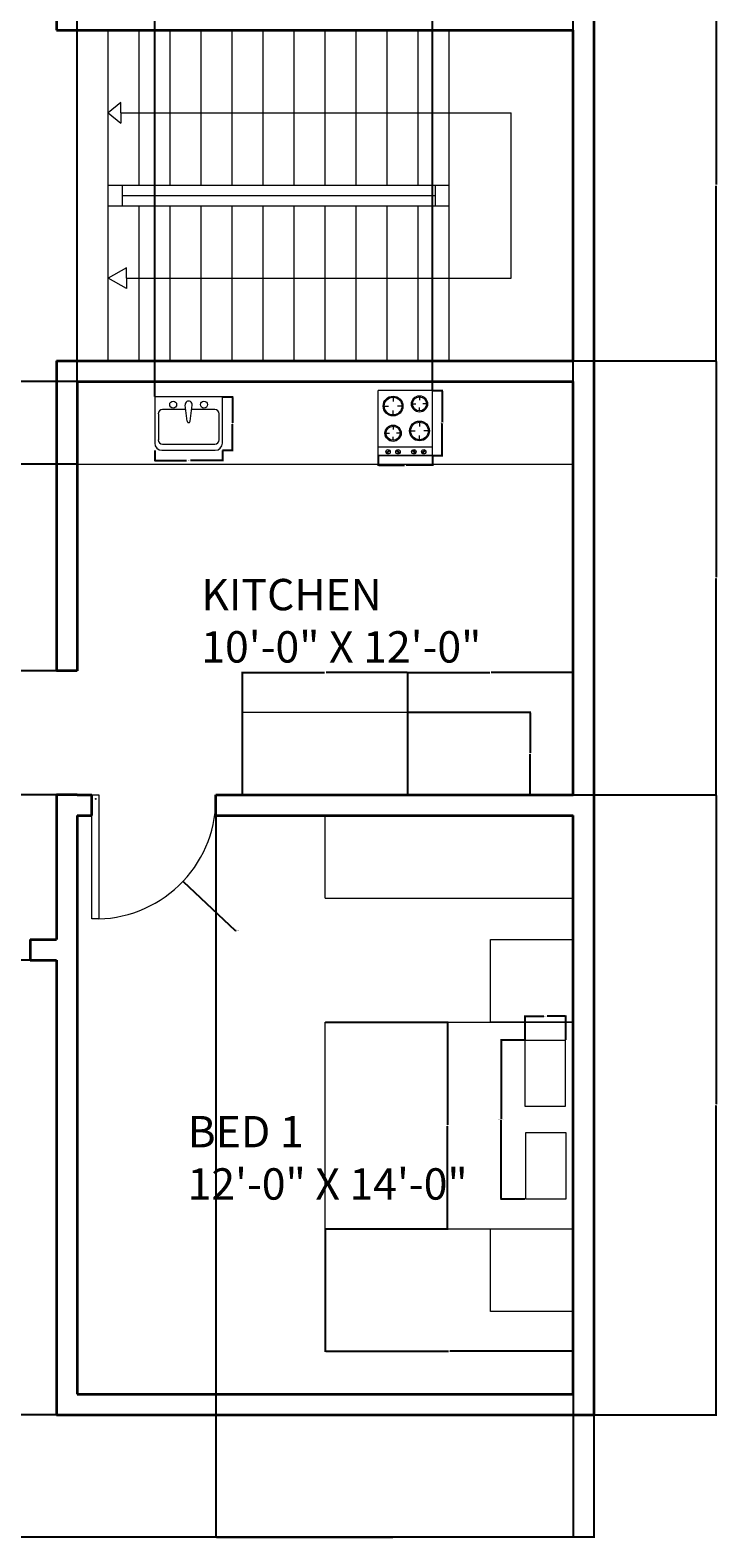
# Model space of a CAD drawing. Units: inches. Extents: x 4468 to 4972, y 2758 to 3538.
# Tile 2 of 4: x 4772 to 4972, y 2758 to 3196. Entities that reach past the tile are written whole.
import ezdxf

# ---------------------------------------------------------------- set-up
doc = ezdxf.new("R2010")
doc.units = ezdxf.units.IN
for name, color, linetype, lineweight in [('A-ANNO-DIMS', 2, 'Continuous', 18), ('A-AREA-IDEN', 7, 'Continuous', 18), ('A-DOOR', 4, 'Continuous', 18), ('A-EQPM', 8, 'Continuous', 18), ('A-FLOR-CASE', 9, 'Continuous', 18), ('A-FLOR-FIXT', 9, 'Continuous', 18), ('A-FLOR-STRS', 3, 'Continuous', 18), ('A-FURN', 8, 'Continuous', 15), ('A-WALL', 7, 'Continuous', 35)]:
    doc.layers.add(name, color=color, linetype=linetype, lineweight=lineweight)
doc.styles.get("Standard").update_dxf_attribs({"font": 'arial.ttf'})
doc.dimstyles.get("Standard").update_dxf_attribs({"dimtxt": 0.18, "dimasz": 0.18, "dimexe": 0.18, "dimexo": 0.0625, "dimgap": 0.09, "dimtad": 0, "dimtih": 1, "dimtoh": 1, "dimdec": 4, "dimzin": 0, "dimdsep": 46, "dimtxsty": 'Standard', "dimcen": 0.09, "dimadec": 0, "dimazin": 0, "dimtfac": 1, "dimtdec": 4, "dimtofl": 0, "dimtmove": 0, "dimatfit": 3, "dimfxl": 1, "dimtolj": 1, "dimtzin": 0, "dimarcsym": 0})

# ---------------------------------------------------------------- blocks, each defined once
blk = doc.blocks.new('A$C16A60262')
at = {"linetype": 'ByBlock'}
for p, q in [((0, 600), (0, 0)), ((488, 600), (0, 600)), ((0, 600), (500, 600)), ((0, 600), (500, 600)), ((500, 600), (500, 0)), ((500, 600), (500, 0)), ((500, 520), (0, 520)), ((119, 456), (119, 415)), ((363, 460), (363, 427)), ((38, 374), (79, 374)), ((119, 293), (119, 334)), ((201, 374), (160, 374)), ((298, 395), (331, 395)), ((363, 330), (363, 362)), ((428, 395), (396, 395)), ((119, 189), (119, 156)), ((282, 144), (323, 144)), ((363, 225), (363, 185)), ((445, 144), (404, 144)), ((0, 0), (500, 0)), ((54, 124), (87, 124)), ((119, 59), (119, 91)), ((184, 124), (152, 124)), ((363, 63), (363, 103))]:
    blk.add_line(p, q, dxfattribs=at)
for p, q in [((66, 557), (87, 579)), ((72, 552), (66, 557)), ((93, 573), (72, 552)), ((87, 579), (93, 573)), ((158, 572), (163, 578)), ((179, 551), (158, 572)), ((163, 578), (184, 557)), ((184, 557), (179, 551)), ((305, 572), (311, 578)), ((326, 551), (305, 572)), ((311, 578), (332, 557)), ((332, 557), (326, 551)), ((396, 558), (417, 580)), ((402, 553), (396, 558)), ((423, 574), (402, 553)), ((417, 580), (423, 574))]:
    blk.add_line(p, q)
for centre in [(80, 566), (171, 566), (318, 566), (409, 566)]:
    blk.add_circle(centre, 20.6)
for centre, radius in [((119, 374), 91.3), ((119, 374), 81.3), ((363, 395), 75), ((363, 395), 65), ((119, 124), 75), ((119, 124), 65), ((363, 144), 91.3), ((363, 144), 81.3)]:
    blk.add_circle(centre, radius, dxfattribs=at)
blk = doc.blocks.new('A$C34D52403')
for p, q in [((0, 0.457), (0, 0.061)), ((0.579, 0.457), (0, 0.457)), ((0.277, 0.249), (0.26, 0.387)), ((0.302, 0.249), (0.319, 0.387)), ((0.579, 0.061), (0.579, 0.457)), ((0.031, 0.312), (0.031, 0.089)), ((0.266, 0.349), (0.068, 0.349)), ((0.513, 0.349), (0.313, 0.349)), ((0.55, 0.089), (0.55, 0.312)), ((0.068, 0.052), (0.513, 0.052)), ((0.061, 0), (0.518, 0))]:
    blk.add_line(p, q)
for centre in [(0.158, 0.391), (0.421, 0.391)]:
    blk.add_circle(centre, 0.0296)
for centre, radius, start, end in [((0.29, 0.391), 0.0296, 353.0422, 186.9578), ((0.068, 0.312), 0.0371, 90, 180), ((0.513, 0.312), 0.0371, 0, 90), ((0.29, 0.249), 0.0125, 179.3528, 0.6472), ((0.061, 0.061), 0.061, 180, 270), ((0.068, 0.089), 0.0371, 180, 270), ((0.513, 0.089), 0.0371, 270, 0), ((0.518, 0.061), 0.061, 270, 0)]:
    blk.add_arc(centre, radius, start, end)
blk = doc.blocks.new('DOOR-LEAF-36IN')
for p, q in [((0, 0), (0, 36)), ((0, 36), (2, 36)), ((2, 36), (2, 0)), ((2, 0), (0, 0))]:
    blk.add_line(p, q)
blk = doc.blocks.new('BED-PILLOW-PAIR')
for points in [[(0, 46.15), (11.65, 46.15), (11.65, 26.85), (0, 26.85)], [(0.18, 19.3), (11.83, 19.3), (11.83, 0), (0.18, 0)]]:
    blk.add_lwpolyline(points, close=True)
blk = doc.blocks.new('NIGHTSTAND-24X24')
blk.add_lwpolyline([(24, 24), (24, 0), (0, 0), (0, 24)], close=True)
blk = doc.blocks.new('*D21')
at = {"layer": 'A-ANNO-DIMS', "color": 0, "lineweight": -2, "transparency": 16777216}
for p, q in [((4916.14, 2902.98), (4909.1, 2902.98)), ((4909.28, 2902.8), (4909.28, 2880.09)), ((4909.28, 2857.01), (4909.28, 2879.72)), ((4916.14, 2856.83), (4909.1, 2856.83))]:
    blk.add_line(p, q, dxfattribs=at)
at = {"layer": 'A-ANNO-DIMS', "color": 0, "transparency": 16777216}
for points in [[(4909.25, 2902.8), (4909.31, 2902.8), (4909.28, 2902.98)], [(4909.25, 2857.01), (4909.31, 2857.01), (4909.28, 2856.83)]]:
    blk.add_solid(points, dxfattribs=at)
at = {"layer": 'Defpoints', "color": 0, "transparency": 16777216}
for p in [(4909.28, 2902.98), (4916.2, 2902.98), (4916.2, 2856.83)]:
    blk.add_point(p, dxfattribs=at)
at = {"layer": 'A-ANNO-DIMS', "color": 0, "transparency": 16777216, "insert": (4909.28, 2879.9), "char_height": 0.18, "attachment_point": 5}
blk.add_mtext('\\A1;PILLOWS 46 TYP.', dxfattribs=at)
blk = doc.blocks.new('*D22')
at = {"layer": 'A-ANNO-DIMS', "color": 0, "lineweight": -2, "transparency": 16777216}
for p, q in [((4916.2, 2903.04), (4916.2, 2910.08)), ((4916.38, 2909.9), (4921.6, 2909.9)), ((4927.85, 2909.9), (4922.63, 2909.9)), ((4928.03, 2903.04), (4928.03, 2910.08))]:
    blk.add_line(p, q, dxfattribs=at)
at = {"layer": 'A-ANNO-DIMS', "color": 0, "transparency": 16777216}
for points in [[(4916.38, 2909.93), (4916.38, 2909.87), (4916.2, 2909.9)], [(4927.85, 2909.93), (4927.85, 2909.87), (4928.03, 2909.9)]]:
    blk.add_solid(points, dxfattribs=at)
at = {"layer": 'Defpoints', "color": 0, "transparency": 16777216}
for p in [(4928.03, 2909.9), (4916.2, 2902.98), (4928.03, 2902.98)]:
    blk.add_point(p, dxfattribs=at)
at = {"layer": 'A-ANNO-DIMS', "color": 0, "transparency": 16777216, "insert": (4922.11, 2909.9), "char_height": 0.18, "attachment_point": 5}
blk.add_mtext('\\A1;12 TYP.', dxfattribs=at)
blk = doc.blocks.new('*D33')
at = {"layer": 'A-ANNO-DIMS', "color": 0, "lineweight": -2, "transparency": 16777216}
for p, q in [((4889.35, 3091.57), (4892.3, 3091.57)), ((4892.12, 3091.39), (4892.12, 3082.31)), ((4892.12, 3072.88), (4892.12, 3081.95)), ((4889.35, 3072.7), (4892.3, 3072.7))]:
    blk.add_line(p, q, dxfattribs=at)
at = {"layer": 'A-ANNO-DIMS', "color": 0, "transparency": 16777216}
for points in [[(4892.09, 3091.39), (4892.15, 3091.39), (4892.12, 3091.57)], [(4892.09, 3072.88), (4892.15, 3072.88), (4892.12, 3072.7)]]:
    blk.add_solid(points, dxfattribs=at)
at = {"layer": 'Defpoints', "color": 0, "transparency": 16777216}
for p in [(4889.29, 3091.57), (4889.29, 3072.7), (4892.12, 3072.7)]:
    blk.add_point(p, dxfattribs=at)
at = {"layer": 'A-ANNO-DIMS', "color": 0, "transparency": 16777216, "insert": (4892.12, 3082.13), "char_height": 0.18, "attachment_point": 5}
blk.add_mtext('\\A1;HOB 19', dxfattribs=at)
blk = doc.blocks.new('*D34')
at = {"layer": 'A-ANNO-DIMS', "color": 0, "lineweight": -2, "transparency": 16777216}
for p, q in [((4873.56, 3072.63), (4873.56, 3069.69)), ((4889.29, 3072.63), (4889.29, 3069.69)), ((4873.74, 3069.87), (4881.22, 3069.87)), ((4889.11, 3069.87), (4881.64, 3069.87))]:
    blk.add_line(p, q, dxfattribs=at)
at = {"layer": 'A-ANNO-DIMS', "color": 0, "transparency": 16777216}
for points in [[(4873.74, 3069.9), (4873.74, 3069.84), (4873.56, 3069.87)], [(4889.11, 3069.9), (4889.11, 3069.84), (4889.29, 3069.87)]]:
    blk.add_solid(points, dxfattribs=at)
at = {"layer": 'Defpoints', "color": 0, "transparency": 16777216}
for p in [(4873.56, 3072.7), (4889.29, 3072.7), (4873.56, 3069.87)]:
    blk.add_point(p, dxfattribs=at)
at = {"layer": 'A-ANNO-DIMS', "color": 0, "transparency": 16777216, "insert": (4881.43, 3069.87), "char_height": 0.18, "attachment_point": 5}
blk.add_mtext('\\A1;16', dxfattribs=at)
blk = doc.blocks.new('*D35')
at = {"layer": 'A-ANNO-DIMS', "color": 0, "lineweight": -2, "transparency": 16777216}
for p, q in [((4808.66, 3074.13), (4808.66, 3071.06)), ((4828.32, 3074.13), (4828.32, 3071.06)), ((4808.84, 3071.24), (4817.94, 3071.24)), ((4828.14, 3071.24), (4819.04, 3071.24))]:
    blk.add_line(p, q, dxfattribs=at)
at = {"layer": 'A-ANNO-DIMS', "color": 0, "transparency": 16777216}
for points in [[(4808.84, 3071.27), (4808.84, 3071.21), (4808.66, 3071.24)], [(4828.14, 3071.27), (4828.14, 3071.21), (4828.32, 3071.24)]]:
    blk.add_solid(points, dxfattribs=at)
at = {"layer": 'Defpoints', "color": 0, "transparency": 16777216}
for p in [(4808.66, 3074.19), (4828.32, 3074.19), (4828.32, 3071.24)]:
    blk.add_point(p, dxfattribs=at)
at = {"layer": 'A-ANNO-DIMS', "color": 0, "transparency": 16777216, "insert": (4818.49, 3071.24), "char_height": 0.18, "attachment_point": 5}
blk.add_mtext('\\A1;SINK 20', dxfattribs=at)
blk = doc.blocks.new('*D36')
at = {"layer": 'A-ANNO-DIMS', "color": 0, "lineweight": -2, "transparency": 16777216}
for p, q in [((4828.38, 3089.71), (4831.45, 3089.71)), ((4831.27, 3089.53), (4831.27, 3082.13)), ((4831.27, 3074.37), (4831.27, 3081.77)), ((4828.38, 3074.19), (4831.45, 3074.19))]:
    blk.add_line(p, q, dxfattribs=at)
at = {"layer": 'A-ANNO-DIMS', "color": 0, "transparency": 16777216}
for points in [[(4831.24, 3089.53), (4831.3, 3089.53), (4831.27, 3089.71)], [(4831.24, 3074.37), (4831.3, 3074.37), (4831.27, 3074.19)]]:
    blk.add_solid(points, dxfattribs=at)
at = {"layer": 'Defpoints', "color": 0, "transparency": 16777216}
for p in [(4828.32, 3089.71), (4831.27, 3089.71), (4828.32, 3074.19)]:
    blk.add_point(p, dxfattribs=at)
at = {"layer": 'A-ANNO-DIMS', "color": 0, "transparency": 16777216, "insert": (4831.27, 3081.95), "char_height": 0.18, "attachment_point": 5}
blk.add_mtext('\\A1;16', dxfattribs=at)
blk = doc.blocks.new('*D37')
at = {"layer": 'A-ANNO-DIMS', "color": 0, "lineweight": -2, "transparency": 16777216}
for p, q in [((4504.18, 2896.1), (4504.18, 2758.48)), ((4936.18, 2794.1), (4936.18, 2758.48)), ((4504.36, 2758.66), (4719.88, 2758.66)), ((4936, 2758.66), (4720.47, 2758.66))]:
    blk.add_line(p, q, dxfattribs=at)
at = {"layer": 'A-ANNO-DIMS', "color": 0, "transparency": 16777216}
for points in [[(4504.36, 2758.69), (4504.36, 2758.63), (4504.18, 2758.66)], [(4936, 2758.69), (4936, 2758.63), (4936.18, 2758.66)]]:
    blk.add_solid(points, dxfattribs=at)
at = {"layer": 'Defpoints', "color": 0, "transparency": 16777216}
for p in [(4504.18, 2896.16), (4936.18, 2794.16), (4936.18, 2758.66)]:
    blk.add_point(p, dxfattribs=at)
at = {"layer": 'A-ANNO-DIMS', "color": 0, "transparency": 16777216, "insert": (4720.18, 2758.66), "char_height": 0.18, "attachment_point": 5}
blk.add_mtext('\\A1;432', dxfattribs=at)
blk = doc.blocks.new('*D38')
at = {"layer": 'A-ANNO-DIMS', "color": 0, "lineweight": -2, "transparency": 16777216}
for p, q in [((4504.11, 3502.16), (4468.5, 3502.16)), ((4468.68, 3501.98), (4468.68, 3148.34)), ((4468.68, 2794.34), (4468.68, 3147.98)), ((4780.11, 2794.16), (4468.5, 2794.16))]:
    blk.add_line(p, q, dxfattribs=at)
at = {"layer": 'A-ANNO-DIMS', "color": 0, "transparency": 16777216}
for points in [[(4468.65, 3501.98), (4468.71, 3501.98), (4468.68, 3502.16)], [(4468.65, 2794.34), (4468.71, 2794.34), (4468.68, 2794.16)]]:
    blk.add_solid(points, dxfattribs=at)
at = {"layer": 'Defpoints', "color": 0, "transparency": 16777216}
for p in [(4468.68, 3502.16), (4504.18, 3502.16), (4780.18, 2794.16)]:
    blk.add_point(p, dxfattribs=at)
at = {"layer": 'A-ANNO-DIMS', "color": 0, "transparency": 16777216, "insert": (4468.68, 3148.16), "char_height": 0.18, "attachment_point": 5}
blk.add_mtext('\\A1;708', dxfattribs=at)
blk = doc.blocks.new('*D42')
at = {"layer": 'A-ANNO-DIMS', "color": 0, "lineweight": -2, "transparency": 16777216}
for p, q in [((4780.11, 2926.16), (4744.5, 2926.16)), ((4744.68, 2925.98), (4744.68, 2860.34)), ((4744.68, 2794.34), (4744.68, 2859.98)), ((4780.11, 2794.16), (4744.5, 2794.16))]:
    blk.add_line(p, q, dxfattribs=at)
at = {"layer": 'A-ANNO-DIMS', "color": 0, "transparency": 16777216}
for points in [[(4744.65, 2925.98), (4744.71, 2925.98), (4744.68, 2926.16)], [(4744.65, 2794.34), (4744.71, 2794.34), (4744.68, 2794.16)]]:
    blk.add_solid(points, dxfattribs=at)
at = {"layer": 'Defpoints', "color": 0, "transparency": 16777216}
for p in [(4744.68, 2926.16), (4780.18, 2926.16), (4780.18, 2794.16)]:
    blk.add_point(p, dxfattribs=at)
at = {"layer": 'A-ANNO-DIMS', "color": 0, "transparency": 16777216, "insert": (4744.68, 2860.16), "char_height": 0.18, "attachment_point": 5}
blk.add_mtext('\\A1;132', dxfattribs=at)
blk = doc.blocks.new('*D45')
at = {"layer": 'A-ANNO-DIMS', "color": 0, "lineweight": -2, "transparency": 16777216}
for p, q in [((4930.24, 3202.16), (4971.86, 3202.16)), ((4971.68, 3201.98), (4971.68, 3151.34)), ((4971.68, 3100.34), (4971.68, 3150.98)), ((4930.24, 3100.16), (4971.86, 3100.16))]:
    blk.add_line(p, q, dxfattribs=at)
at = {"layer": 'A-ANNO-DIMS', "color": 0, "transparency": 16777216}
for points in [[(4971.65, 3201.98), (4971.71, 3201.98), (4971.68, 3202.16)], [(4971.65, 3100.34), (4971.71, 3100.34), (4971.68, 3100.16)]]:
    blk.add_solid(points, dxfattribs=at)
at = {"layer": 'Defpoints', "color": 0, "transparency": 16777216}
for p in [(4930.18, 3202.16), (4971.68, 3202.16), (4930.18, 3100.16)]:
    blk.add_point(p, dxfattribs=at)
at = {"layer": 'A-ANNO-DIMS', "color": 0, "transparency": 16777216, "insert": (4971.68, 3151.16), "char_height": 0.18, "attachment_point": 5}
blk.add_mtext('\\A1;102', dxfattribs=at)
blk = doc.blocks.new('*D46')
at = {"layer": 'A-ANNO-DIMS', "color": 0, "lineweight": -2, "transparency": 16777216}
for p, q in [((4930.24, 3100.16), (4971.86, 3100.16)), ((4971.68, 3099.98), (4971.68, 3037.34)), ((4971.68, 2974.34), (4971.68, 3036.98)), ((4930.24, 2974.16), (4971.86, 2974.16))]:
    blk.add_line(p, q, dxfattribs=at)
at = {"layer": 'A-ANNO-DIMS', "color": 0, "transparency": 16777216}
for points in [[(4971.65, 3099.98), (4971.71, 3099.98), (4971.68, 3100.16)], [(4971.65, 2974.34), (4971.71, 2974.34), (4971.68, 2974.16)]]:
    blk.add_solid(points, dxfattribs=at)
at = {"layer": 'Defpoints', "color": 0, "transparency": 16777216}
for p in [(4930.18, 3100.16), (4971.68, 3100.16), (4930.18, 2974.16)]:
    blk.add_point(p, dxfattribs=at)
at = {"layer": 'A-ANNO-DIMS', "color": 0, "transparency": 16777216, "insert": (4971.68, 3037.16), "char_height": 0.18, "attachment_point": 5}
blk.add_mtext('\\A1;126', dxfattribs=at)
blk = doc.blocks.new('*D47')
at = {"layer": 'A-ANNO-DIMS', "color": 0, "lineweight": -2, "transparency": 16777216}
for p, q in [((4930.24, 2974.16), (4971.86, 2974.16)), ((4971.68, 2973.98), (4971.68, 2884.34)), ((4971.68, 2794.34), (4971.68, 2883.98)), ((4936.24, 2794.16), (4971.86, 2794.16))]:
    blk.add_line(p, q, dxfattribs=at)
at = {"layer": 'A-ANNO-DIMS', "color": 0, "transparency": 16777216}
for points in [[(4971.65, 2973.98), (4971.71, 2973.98), (4971.68, 2974.16)], [(4971.65, 2794.34), (4971.71, 2794.34), (4971.68, 2794.16)]]:
    blk.add_solid(points, dxfattribs=at)
at = {"layer": 'Defpoints', "color": 0, "transparency": 16777216}
for p in [(4930.18, 2974.16), (4971.68, 2974.16), (4936.18, 2794.16)]:
    blk.add_point(p, dxfattribs=at)
at = {"layer": 'A-ANNO-DIMS', "color": 0, "transparency": 16777216, "insert": (4971.68, 2884.16), "char_height": 0.18, "attachment_point": 5}
blk.add_mtext('\\A1;180', dxfattribs=at)
blk = doc.blocks.new('*D55')
at = {"layer": 'A-ANNO-DIMS', "color": 0, "lineweight": -2, "transparency": 16777216}
for p, q in [((4786.11, 3094.16), (4468.5, 3094.16)), ((4468.68, 3093.98), (4468.68, 3082.34)), ((4468.68, 3070.34), (4468.68, 3081.98)), ((4786.11, 3070.16), (4468.5, 3070.16))]:
    blk.add_line(p, q, dxfattribs=at)
at = {"layer": 'A-ANNO-DIMS', "color": 0, "transparency": 16777216}
for points in [[(4468.65, 3093.98), (4468.71, 3093.98), (4468.68, 3094.16)], [(4468.65, 3070.34), (4468.71, 3070.34), (4468.68, 3070.16)]]:
    blk.add_solid(points, dxfattribs=at)
at = {"layer": 'Defpoints', "color": 0, "transparency": 16777216}
for p in [(4468.68, 3094.16), (4786.18, 3094.16), (4786.18, 3070.16)]:
    blk.add_point(p, dxfattribs=at)
at = {"layer": 'A-ANNO-DIMS', "color": 0, "transparency": 16777216, "insert": (4468.68, 3082.16), "char_height": 0.18, "attachment_point": 5}
blk.add_mtext('\\A1;24', dxfattribs=at)
blk = doc.blocks.new('*D56')
at = {"layer": 'A-ANNO-DIMS', "color": 0, "lineweight": -2, "transparency": 16777216}
for p, q in [((4786.11, 3010.16), (4468.5, 3010.16)), ((4468.68, 3009.98), (4468.68, 2992.34)), ((4468.68, 2974.34), (4468.68, 2991.98)), ((4786.11, 2974.16), (4468.5, 2974.16))]:
    blk.add_line(p, q, dxfattribs=at)
at = {"layer": 'A-ANNO-DIMS', "color": 0, "transparency": 16777216}
for points in [[(4468.65, 3009.98), (4468.71, 3009.98), (4468.68, 3010.16)], [(4468.65, 2974.34), (4468.71, 2974.34), (4468.68, 2974.16)]]:
    blk.add_solid(points, dxfattribs=at)
at = {"layer": 'Defpoints', "color": 0, "transparency": 16777216}
for p in [(4468.68, 3010.16), (4786.18, 3010.16), (4786.18, 2974.16)]:
    blk.add_point(p, dxfattribs=at)
at = {"layer": 'A-ANNO-DIMS', "color": 0, "transparency": 16777216, "insert": (4468.68, 2992.16), "char_height": 0.18, "attachment_point": 5}
blk.add_mtext('\\A1;36', dxfattribs=at)
blk = doc.blocks.new('*D59')
at = {"layer": 'A-ANNO-DIMS', "color": 0, "lineweight": -2, "transparency": 16777216}
for p, q in [((4858.24, 2908.16), (4893.86, 2908.16)), ((4893.68, 2907.98), (4893.68, 2878.34)), ((4893.68, 2848.34), (4893.68, 2877.98)), ((4858.24, 2848.16), (4893.86, 2848.16))]:
    blk.add_line(p, q, dxfattribs=at)
at = {"layer": 'A-ANNO-DIMS', "color": 0, "transparency": 16777216}
for points in [[(4893.65, 2907.98), (4893.71, 2907.98), (4893.68, 2908.16)], [(4893.65, 2848.34), (4893.71, 2848.34), (4893.68, 2848.16)]]:
    blk.add_solid(points, dxfattribs=at)
at = {"layer": 'Defpoints', "color": 0, "transparency": 16777216}
for p in [(4858.18, 2908.16), (4858.18, 2848.16), (4893.68, 2848.16)]:
    blk.add_point(p, dxfattribs=at)
at = {"layer": 'A-ANNO-DIMS', "color": 0, "transparency": 16777216, "insert": (4893.68, 2878.16), "char_height": 0.18, "attachment_point": 5}
blk.add_mtext('\\A1;60', dxfattribs=at)
blk = doc.blocks.new('*D60')
at = {"layer": 'A-ANNO-DIMS', "color": 0, "lineweight": -2, "transparency": 16777216}
for p, q in [((4858.18, 2848.1), (4858.18, 2812.48)), ((4930.18, 2848.1), (4930.18, 2812.48)), ((4858.36, 2812.66), (4893.96, 2812.66)), ((4930, 2812.66), (4894.39, 2812.66))]:
    blk.add_line(p, q, dxfattribs=at)
at = {"layer": 'A-ANNO-DIMS', "color": 0, "transparency": 16777216}
for points in [[(4858.36, 2812.69), (4858.36, 2812.63), (4858.18, 2812.66)], [(4930, 2812.69), (4930, 2812.63), (4930.18, 2812.66)]]:
    blk.add_solid(points, dxfattribs=at)
at = {"layer": 'Defpoints', "color": 0, "transparency": 16777216}
for p in [(4858.18, 2848.16), (4930.18, 2848.16), (4858.18, 2812.66)]:
    blk.add_point(p, dxfattribs=at)
at = {"layer": 'A-ANNO-DIMS', "color": 0, "transparency": 16777216, "insert": (4894.18, 2812.66), "char_height": 0.18, "attachment_point": 5}
blk.add_mtext('\\A1;72', dxfattribs=at)
blk = doc.blocks.new('*D65')
at = {"layer": 'A-ANNO-DIMS', "color": 0, "lineweight": -2, "transparency": 16777216}
for p, q in [((4826.4, 2968.1), (4826.4, 2758.48)), ((4930.18, 2968.1), (4930.18, 2758.48)), ((4826.58, 2758.66), (4877.83, 2758.66)), ((4930, 2758.66), (4878.74, 2758.66))]:
    blk.add_line(p, q, dxfattribs=at)
at = {"layer": 'A-ANNO-DIMS', "color": 0, "transparency": 16777216}
for points in [[(4826.58, 2758.69), (4826.58, 2758.63), (4826.4, 2758.66)], [(4930, 2758.69), (4930, 2758.63), (4930.18, 2758.66)]]:
    blk.add_solid(points, dxfattribs=at)
at = {"layer": 'Defpoints', "color": 0, "transparency": 16777216}
for p in [(4826.4, 2968.16), (4930.18, 2968.16), (4930.18, 2758.66)]:
    blk.add_point(p, dxfattribs=at)
at = {"layer": 'A-ANNO-DIMS', "color": 0, "transparency": 16777216, "insert": (4878.29, 2758.66), "char_height": 0.18, "attachment_point": 5}
blk.add_mtext('\\A1;103.77', dxfattribs=at)
blk = doc.blocks.new('*D70')
at = {"layer": 'A-ANNO-DIMS', "color": 0, "lineweight": -2, "transparency": 16777216}
for p, q in [((4786.18, 3094.22), (4786.18, 3537.84)), ((4786.36, 3537.66), (4796.95, 3537.66)), ((4808.48, 3537.66), (4797.88, 3537.66)), ((4808.66, 3089.77), (4808.66, 3537.84))]:
    blk.add_line(p, q, dxfattribs=at)
at = {"layer": 'A-ANNO-DIMS', "color": 0, "transparency": 16777216}
for points in [[(4786.36, 3537.69), (4786.36, 3537.63), (4786.18, 3537.66)], [(4808.48, 3537.69), (4808.48, 3537.63), (4808.66, 3537.66)]]:
    blk.add_solid(points, dxfattribs=at)
at = {"layer": 'Defpoints', "color": 0, "transparency": 16777216}
for p in [(4808.66, 3537.66), (4786.18, 3094.16), (4808.66, 3089.71)]:
    blk.add_point(p, dxfattribs=at)
at = {"layer": 'A-ANNO-DIMS', "color": 0, "transparency": 16777216, "insert": (4797.42, 3537.66), "char_height": 0.18, "attachment_point": 5}
blk.add_mtext('\\A1;22.487', dxfattribs=at)
blk = doc.blocks.new('*D71')
at = {"layer": 'A-ANNO-DIMS', "color": 0, "lineweight": -2, "transparency": 16777216}
for p, q in [((4889.29, 3091.63), (4889.29, 3537.84)), ((4889.47, 3537.66), (4909.33, 3537.66)), ((4930, 3537.66), (4910.13, 3537.66)), ((4930.18, 3094.22), (4930.18, 3537.84))]:
    blk.add_line(p, q, dxfattribs=at)
at = {"layer": 'A-ANNO-DIMS', "color": 0, "transparency": 16777216}
for points in [[(4889.47, 3537.69), (4889.47, 3537.63), (4889.29, 3537.66)], [(4930, 3537.69), (4930, 3537.63), (4930.18, 3537.66)]]:
    blk.add_solid(points, dxfattribs=at)
at = {"layer": 'Defpoints', "color": 0, "transparency": 16777216}
for p in [(4930.18, 3537.66), (4889.29, 3091.57), (4930.18, 3094.16)]:
    blk.add_point(p, dxfattribs=at)
at = {"layer": 'A-ANNO-DIMS', "color": 0, "transparency": 16777216, "insert": (4909.73, 3537.66), "char_height": 0.18, "attachment_point": 5}
blk.add_mtext('\\A1;40.89', dxfattribs=at)
blk = doc.blocks.new('*D72')
at = {"layer": 'A-ANNO-DIMS', "color": 0, "lineweight": -2, "transparency": 16777216}
for p, q in [((4834.18, 2974.22), (4834.18, 3009.84)), ((4834.36, 3009.66), (4857.95, 3009.66)), ((4882, 3009.66), (4858.4, 3009.66)), ((4882.18, 2974.22), (4882.18, 3009.84))]:
    blk.add_line(p, q, dxfattribs=at)
at = {"layer": 'A-ANNO-DIMS', "color": 0, "transparency": 16777216}
for points in [[(4834.36, 3009.69), (4834.36, 3009.63), (4834.18, 3009.66)], [(4882, 3009.69), (4882, 3009.63), (4882.18, 3009.66)]]:
    blk.add_solid(points, dxfattribs=at)
at = {"layer": 'Defpoints', "color": 0, "transparency": 16777216}
for p in [(4882.18, 3009.66), (4834.18, 2974.16), (4882.18, 2974.16)]:
    blk.add_point(p, dxfattribs=at)
at = {"layer": 'A-ANNO-DIMS', "color": 0, "transparency": 16777216, "insert": (4858.18, 3009.66), "char_height": 0.18, "attachment_point": 5}
blk.add_mtext('\\A1;48', dxfattribs=at)
blk = doc.blocks.new('*D73')
at = {"layer": 'A-ANNO-DIMS', "color": 0, "lineweight": -2, "transparency": 16777216}
for p, q in [((4882.24, 2998.16), (4917.86, 2998.16)), ((4917.68, 2997.98), (4917.68, 2986.34)), ((4917.68, 2974.34), (4917.68, 2985.98)), ((4882.24, 2974.16), (4917.86, 2974.16))]:
    blk.add_line(p, q, dxfattribs=at)
at = {"layer": 'A-ANNO-DIMS', "color": 0, "transparency": 16777216}
for points in [[(4917.65, 2997.98), (4917.71, 2997.98), (4917.68, 2998.16)], [(4917.65, 2974.34), (4917.71, 2974.34), (4917.68, 2974.16)]]:
    blk.add_solid(points, dxfattribs=at)
at = {"layer": 'Defpoints', "color": 0, "transparency": 16777216}
for p in [(4882.18, 2998.16), (4882.18, 2974.16), (4917.68, 2974.16)]:
    blk.add_point(p, dxfattribs=at)
at = {"layer": 'A-ANNO-DIMS', "color": 0, "transparency": 16777216, "insert": (4917.68, 2986.16), "char_height": 0.18, "attachment_point": 5}
blk.add_mtext('\\A1;24', dxfattribs=at)
blk = doc.blocks.new('*D74')
at = {"layer": 'A-ANNO-DIMS', "color": 0, "lineweight": -2, "transparency": 16777216}
for p, q in [((4882.18, 2974.22), (4882.18, 3009.84)), ((4882.36, 3009.66), (4905.95, 3009.66)), ((4930, 3009.66), (4906.4, 3009.66)), ((4930.18, 2974.22), (4930.18, 3009.84))]:
    blk.add_line(p, q, dxfattribs=at)
at = {"layer": 'A-ANNO-DIMS', "color": 0, "transparency": 16777216}
for points in [[(4882.36, 3009.69), (4882.36, 3009.63), (4882.18, 3009.66)], [(4930, 3009.69), (4930, 3009.63), (4930.18, 3009.66)]]:
    blk.add_solid(points, dxfattribs=at)
at = {"layer": 'Defpoints', "color": 0, "transparency": 16777216}
for p in [(4930.18, 3009.66), (4882.18, 2974.16), (4930.18, 2974.16)]:
    blk.add_point(p, dxfattribs=at)
at = {"layer": 'A-ANNO-DIMS', "color": 0, "transparency": 16777216, "insert": (4906.18, 3009.66), "char_height": 0.18, "attachment_point": 5}
blk.add_mtext('\\A1;48', dxfattribs=at)
blk = doc.blocks.new('*D78')
at = {"layer": 'A-ANNO-DIMS', "color": 0, "lineweight": -2, "transparency": 16777216}
for p, q in [((4791.45, 2973.03), (4791.63, 2973.03)), ((4791.54, 2972.94), (4791.54, 2973.12)), ((4832.12, 2934.71), (4817.03, 2948.95)), ((4832.3, 2934.71), (4832.12, 2934.71))]:
    blk.add_line(p, q, dxfattribs=at)
at = {"layer": 'A-ANNO-DIMS', "color": 0, "transparency": 16777216}
blk.add_solid([(4817.05, 2948.98), (4817.01, 2948.93), (4816.9, 2949.08)], dxfattribs=at)
at = {"layer": 'Defpoints', "color": 0, "transparency": 16777216}
for p in [(4791.54, 2973.03), (4816.9, 2949.08)]:
    blk.add_point(p, dxfattribs=at)
at = {"layer": 'A-ANNO-DIMS', "color": 0, "transparency": 16777216, "insert": (4832.78, 2934.71), "char_height": 0.18, "attachment_point": 5}
blk.add_mtext('\\A1;R34.88', dxfattribs=at)

msp = doc.modelspace()

# ---------------------------------------------------------------- linework, layer by layer
at = {"layer": 'A-DOOR'}
msp.add_arc((4791.5442, 2973.0257), 34.8781, 271.412367, 1.860787, dxfattribs=at)
at = {"layer": 'A-FLOR-CASE'}
for p, q in [((4786.1753, 3070.1582), (4930.1753, 3070.1582)), ((4834.1753, 2974.1582), (4834.1753, 2998.1582)), ((4834.1753, 2998.1582), (4882.1753, 2998.1582)), ((4882.1753, 2974.1582), (4882.1753, 2998.1582)), ((4858.1753, 2944.1582), (4858.1753, 2968.1582)), ((4858.1753, 2944.1582), (4930.1753, 2944.1582))]:
    msp.add_line(p, q, dxfattribs=at)
at = {"layer": 'A-FLOR-STRS'}
for p, q in [((4795.1753, 3100.1582), (4795.1753, 3196.1582)), ((4804.1753, 3151.1582), (4804.1753, 3196.1582)), ((4813.1753, 3151.1582), (4813.1753, 3196.1582)), ((4822.1753, 3151.1582), (4822.1753, 3196.1582)), ((4831.1753, 3151.1582), (4831.1753, 3196.1582)), ((4840.1753, 3151.1582), (4840.1753, 3196.1582)), ((4849.1753, 3151.1582), (4849.1753, 3196.1582)), ((4858.1753, 3151.1582), (4858.1753, 3196.1582)), ((4867.1753, 3151.1582), (4867.1753, 3196.1582)), ((4876.1753, 3151.1582), (4876.1753, 3196.1582)), ((4885.1753, 3151.1582), (4885.1753, 3196.1582)), ((4894.1753, 3100.1582), (4894.1753, 3196.1582)), ((4798.8526, 3175.1582), (4795.1753, 3172.1582)), ((4798.8526, 3172.1582), (4798.8526, 3175.1582)), ((4795.1753, 3172.1582), (4798.8526, 3169.1582)), ((4798.8526, 3172.1582), (4912.1753, 3172.1582)), ((4798.8526, 3172.1582), (4798.8526, 3169.1582)), ((4912.1753, 3124.1582), (4912.1753, 3172.1582)), ((4795.1753, 3151.1582), (4894.1753, 3151.1582)), ((4799.1912, 3151.1582), (4799.1912, 3145.1582)), ((4799.1912, 3148.1582), (4890.1306, 3148.1582)), ((4890.1306, 3151.1582), (4890.1306, 3145.1582)), ((4795.1753, 3145.1582), (4894.1753, 3145.1582)), ((4804.1753, 3100.1582), (4804.1753, 3145.1582)), ((4813.1753, 3100.1582), (4813.1753, 3145.1582)), ((4822.1753, 3100.1582), (4822.1753, 3145.1582)), ((4831.1753, 3100.1582), (4831.1753, 3145.1582)), ((4840.1753, 3100.1582), (4840.1753, 3145.1582)), ((4849.1753, 3100.1582), (4849.1753, 3145.1582)), ((4858.1753, 3100.1582), (4858.1753, 3145.1582)), ((4867.1753, 3100.1582), (4867.1753, 3145.1582)), ((4876.1753, 3100.1582), (4876.1753, 3145.1582)), ((4885.1753, 3100.1582), (4885.1753, 3145.1582)), ((4800.4723, 3127.1582), (4795.1753, 3124.1582)), ((4800.4723, 3124.1582), (4800.4723, 3127.1582)), ((4800.4723, 3121.1582), (4795.1753, 3124.1582)), ((4800.4723, 3124.1582), (4912.1753, 3124.1582)), ((4800.4723, 3124.1582), (4800.4723, 3121.1582))]:
    msp.add_line(p, q, dxfattribs=at)
at = {"layer": 'A-FURN'}
for p, q in [((4858.1753, 2848.1582), (4858.1753, 2908.1582)), ((4858.1753, 2908.1582), (4930.1753, 2908.1582)), ((4858.1753, 2848.1582), (4930.1753, 2848.1582))]:
    msp.add_line(p, q, dxfattribs=at)
at = {"layer": 'A-WALL'}
for p, q in [((4936.1753, 3502.1582), (4936.1753, 2794.1582)), ((4780.1753, 3305.7201), (4780.1753, 3196.1582)), ((4780.1753, 3196.1582), (4930.1753, 3196.1582)), ((4930.1753, 3100.1582), (4930.1753, 3196.1582)), ((4780.1753, 3100.1582), (4930.1753, 3100.1582)), ((4780.1753, 3100.1582), (4780.1753, 3010.1582)), ((4786.1753, 3094.1582), (4930.1753, 3094.1582)), ((4786.1753, 3094.1582), (4786.1753, 3010.1582)), ((4930.1753, 2974.1582), (4930.1753, 3094.1582)), ((4786.1753, 3010.1582), (4780.1753, 3010.1582)), ((4786.1753, 2974.1582), (4780.1753, 2974.1582)), ((4780.1753, 2974.1582), (4780.1753, 2932.1582)), ((4786.1753, 2974.1582), (4790.4039, 2974.1582)), ((4790.4039, 2968.1582), (4790.4039, 2974.1582)), ((4826.4039, 2968.1582), (4826.4039, 2974.1582)), ((4826.4039, 2974.1582), (4930.1753, 2974.1582)), ((4786.1753, 2968.1582), (4790.4039, 2968.1582)), ((4786.1753, 2968.1582), (4786.1753, 2800.1582)), ((4826.4039, 2968.1582), (4930.1753, 2968.1582)), ((4930.1753, 2800.1582), (4930.1753, 2968.1582)), ((4772.4962, 2932.1582), (4772.4962, 2926.1582)), ((4772.4962, 2932.1582), (4780.1753, 2932.1582)), ((4772.4962, 2926.1582), (4780.1753, 2926.1582)), ((4780.1753, 2926.1582), (4780.1753, 2794.1582)), ((4786.1753, 2800.1582), (4930.1753, 2800.1582)), ((4780.1753, 2794.1582), (4936.1753, 2794.1582))]:
    msp.add_line(p, q, dxfattribs=at)

# ---------------------------------------------------------------- block references
at = {"layer": 'A-DOOR'}
msp.add_blockref('DOOR-LEAF-36IN', (4790.4039, 2938.1582), dxfattribs=at)
at = {"layer": 'A-EQPM', "xscale": 0.0314475394967079, "yscale": 0.0314475394967079, "zscale": 0.0314475394967079, "rotation": 179.9999999999991}
msp.add_blockref('A$C16A60262', (4889.2887, 3091.5651), dxfattribs=at)
at = {"layer": 'A-FLOR-FIXT', "xscale": 33.94412618968887, "yscale": 33.94412618968887, "zscale": 33.94412618968887}
msp.add_blockref('A$C34D52403', (4808.6626, 3074.1915), dxfattribs=at)
at = {"layer": 'A-FURN'}
for name, p in [('NIGHTSTAND-24X24', (4906.1753, 2908.1582)), ('BED-PILLOW-PAIR', (4916.2002, 2856.8287)), ('NIGHTSTAND-24X24', (4906.1753, 2824.1582))]:
    msp.add_blockref(name, p, dxfattribs=at)

# ---------------------------------------------------------------- texts
at = {"layer": 'A-AREA-IDEN', "char_height": 9.103585, "attachment_point": 1}
for s, insert in [('KITCHEN\\P10\'-0" X 12\'-0"', (4822.1796, 3036.8545)), ('BED 1\\P12\'-0" X 14\'-0"', (4818.2063, 2880.9412))]:
    msp.add_mtext_dynamic_manual_height_columns(s, width=327.642018, gutter_width=45.5179, heights=[0], dxfattribs=dict(at, insert=insert))

# ---------------------------------------------------------------- dimensions: what is measured, and where the dimension line sits
at = {"layer": 'A-ANNO-DIMS'}
for base, p1, p2, override, picture, middle in [((4808.6626, 3537.6582), (4786.1753, 3094.1582), (4808.6626, 3089.7108), {"dimdec": 3, "dimlfac": 1, "dimrnd": 0, "dimzin": 0, "dimdsep": 46, "dimlunit": 2}, '*D70', (4797.4189, 3537.6582)), ((4930.1753, 3537.6582), (4889.2887, 3091.5651), (4930.1753, 3094.1582), {"dimdec": 2, "dimlfac": 1, "dimrnd": 0, "dimzin": 0, "dimdsep": 46, "dimlunit": 2}, '*D71', (4909.732, 3537.6582)), ((4882.1753, 3009.6582), (4834.1753, 2974.1582), (4882.1753, 2974.1582), {"dimdec": 0, "dimlfac": 1, "dimrnd": 0, "dimzin": 0, "dimdsep": 46, "dimlunit": 2}, '*D72', (4858.1753, 3009.6582)), ((4930.1753, 3009.6582), (4882.1753, 2974.1582), (4930.1753, 2974.1582), {"dimdec": 0, "dimlfac": 1, "dimrnd": 0, "dimzin": 0, "dimdsep": 46, "dimlunit": 2}, '*D74', (4906.1753, 3009.6582)), ((4930.1753, 2758.6582), (4826.4039, 2968.1582), (4930.1753, 2968.1582), {"dimdec": 2, "dimlfac": 1, "dimrnd": 0, "dimzin": 0, "dimdsep": 46, "dimlunit": 2}, '*D65', (4878.2896, 2758.6582)), ((4936.1753, 2758.6582), (4504.1753, 2896.1582), (4936.1753, 2794.1582), {"dimdec": 0, "dimlfac": 1, "dimrnd": 0, "dimzin": 0, "dimdsep": 46, "dimlunit": 2}, '*D37', (4720.1753, 2758.6582))]:
    dim = msp.add_linear_dim(base=base, p1=p1, p2=p2, dimstyle='Standard', override=override, dxfattribs=at)
    dim.commit()
    dim.dimension.update_dxf_attribs({"geometry": picture, "text_midpoint": middle})
for base, p1, p2, angle, picture, middle in [((4468.6753, 3502.1582), (4780.1753, 2794.1582), (4504.1753, 3502.1582), 90, '*D38', (4468.6753, 3148.1582)), ((4971.6753, 3202.1582), (4930.1753, 3100.1582), (4930.1753, 3202.1582), 90, '*D45', (4971.6753, 3151.1582)), ((4971.6753, 3100.1582), (4930.1753, 2974.1582), (4930.1753, 3100.1582), 90, '*D46', (4971.6753, 3037.1582)), ((4468.6753, 3094.1582), (4786.1753, 3070.1582), (4786.1753, 3094.1582), 90, '*D55', (4468.6753, 3082.1582)), ((4831.2689, 3089.7108), (4828.3203, 3074.1915), (4828.3203, 3089.7108), 90, '*D36', (4831.2689, 3081.9512)), ((4873.5649, 3069.8663), (4889.2887, 3072.6965), (4873.5649, 3072.6965), 180, '*D34', (4881.4268, 3069.8663)), ((4468.6753, 3010.1582), (4786.1753, 2974.1582), (4786.1753, 3010.1582), 90, '*D56', (4468.6753, 2992.1582)), ((4917.6753, 2974.1582), (4882.1753, 2998.1582), (4882.1753, 2974.1582), 270, '*D73', (4917.6753, 2986.1582)), ((4971.6753, 2974.1582), (4936.1753, 2794.1582), (4930.1753, 2974.1582), 90, '*D47', (4971.6753, 2884.1582)), ((4744.6753, 2926.1582), (4780.1753, 2794.1582), (4780.1753, 2926.1582), 90, '*D42', (4744.6753, 2860.1582)), ((4893.6753, 2848.1582), (4858.1753, 2908.1582), (4858.1753, 2848.1582), 270, '*D59', (4893.6753, 2878.1582)), ((4858.1753, 2812.6582), (4930.1753, 2848.1582), (4858.1753, 2848.1582), 180, '*D60', (4894.1753, 2812.6582))]:
    dim = msp.add_linear_dim(base=base, p1=p1, p2=p2, angle=angle, dimstyle='Standard', override={"dimdec": 0, "dimlfac": 1, "dimrnd": 0, "dimzin": 0, "dimdsep": 46, "dimlunit": 2}, dxfattribs=at)
    dim.commit()
    dim.dimension.update_dxf_attribs({"geometry": picture, "text_midpoint": middle})
for base, p1, p2, angle, text, picture, middle in [((4892.1189, 3072.6965), (4889.2887, 3091.5651), (4889.2887, 3072.6965), 270, 'HOB <>', '*D33', (4892.1189, 3082.1308)), ((4909.2779, 2902.9775), (4916.2002, 2856.8287), (4916.2002, 2902.9775), 90, 'PILLOWS <> TYP.', '*D21', (4909.2779, 2879.9031))]:
    dim = msp.add_linear_dim(base=base, p1=p1, p2=p2, angle=angle, text=text, dimstyle='Standard', override={"dimdec": 0, "dimlfac": 1, "dimrnd": 0, "dimzin": 0, "dimdsep": 46, "dimlunit": 2}, dxfattribs=at)
    dim.commit()
    dim.dimension.update_dxf_attribs({"geometry": picture, "text_midpoint": middle})
for base, p1, p2, text, picture, middle in [((4828.3203, 3071.2429), (4808.6626, 3074.1915), (4828.3203, 3074.1915), 'SINK <>', '*D35', (4818.4914, 3071.2429)), ((4928.0292, 2909.8998), (4916.2002, 2902.9775), (4928.0292, 2902.9775), '<> TYP.', '*D22', (4922.1147, 2909.8998))]:
    dim = msp.add_linear_dim(base=base, p1=p1, p2=p2, text=text, dimstyle='Standard', override={"dimdec": 0, "dimlfac": 1, "dimrnd": 0, "dimzin": 0, "dimdsep": 46, "dimlunit": 2}, dxfattribs=at)
    dim.commit()
    dim.dimension.update_dxf_attribs({"geometry": picture, "text_midpoint": middle})
dim = msp.add_radius_dim(center=(4791.5442, 2973.0257), mpoint=(4816.9012, 2949.0778), dimstyle='Standard', override={"dimdec": 2, "dimlfac": 1, "dimrnd": 0, "dimzin": 0, "dimdsep": 46, "dimlunit": 2}, dxfattribs=at)
dim.commit()
dim.dimension.update_dxf_attribs({"geometry": '*D78', "text_midpoint": (4832.7754, 2934.7091), "dimtype": 164})

doc.saveas('drawing.dxf')
